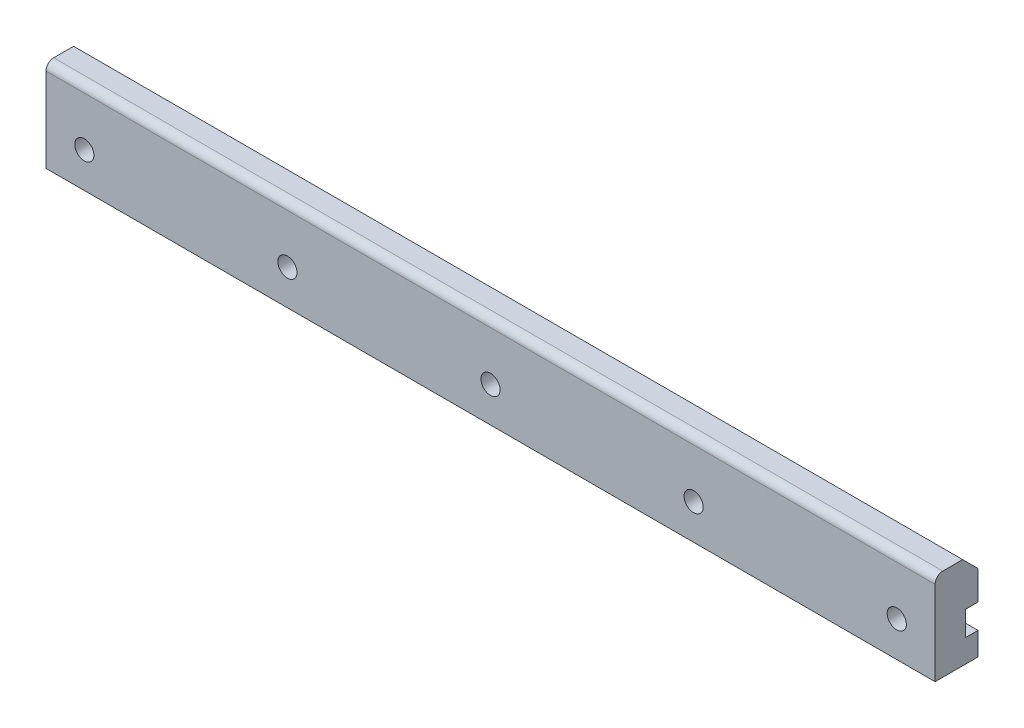
ISO-10303-21;
HEADER;
FILE_DESCRIPTION(('STEP AP214'),'2;1');
FILE_NAME('part.step','',(''),(''),'','','');
FILE_SCHEMA(('AUTOMOTIVE_DESIGN { 1 0 10303 214 1 1 1 1 }'));
ENDSEC;
DATA;
#1=APPLICATION_CONTEXT('core data for automotive mechanical design processes');
#2=APPLICATION_PROTOCOL_DEFINITION('international standard','automotive_design',2000,#1);
#3=PRODUCT_CONTEXT('',#1,'mechanical');
#4=PRODUCT('Part','Part','',(#3));
#5=PRODUCT_RELATED_PRODUCT_CATEGORY('part','',(#4));
#6=PRODUCT_DEFINITION_FORMATION('','',#4);
#7=PRODUCT_DEFINITION_CONTEXT('part definition',#1,'design');
#8=PRODUCT_DEFINITION('design','',#6,#7);
#9=PRODUCT_DEFINITION_SHAPE('','',#8);
#10=(LENGTH_UNIT() NAMED_UNIT(*) SI_UNIT(.MILLI.,.METRE.));
#11=(NAMED_UNIT(*) PLANE_ANGLE_UNIT() SI_UNIT($,.RADIAN.));
#12=(NAMED_UNIT(*) SI_UNIT($,.STERADIAN.) SOLID_ANGLE_UNIT());
#13=UNCERTAINTY_MEASURE_WITH_UNIT(LENGTH_MEASURE(1.E-05),#10,'distance_accuracy_value','');
#14=(GEOMETRIC_REPRESENTATION_CONTEXT(3) GLOBAL_UNCERTAINTY_ASSIGNED_CONTEXT((#13)) GLOBAL_UNIT_ASSIGNED_CONTEXT((#10,
#11,#12)) REPRESENTATION_CONTEXT('',''));
#15=CARTESIAN_POINT('',(0.,0.,0.));
#16=DIRECTION('',(0.,0.,1.));
#17=DIRECTION('',(1.,0.,0.));
#18=AXIS2_PLACEMENT_3D('',#15,#16,#17);
#19=CARTESIAN_POINT('',(0.,0.,0.));
#20=DIRECTION('',(0.,0.,1.));
#21=DIRECTION('',(1.,0.,0.));
#22=AXIS2_PLACEMENT_3D('',#19,#20,#21);
#23=PLANE('',#22);
#24=DIRECTION('',(0.,-1.,0.));
#25=VECTOR('',#24,1.);
#26=CARTESIAN_POINT('',(-290.,30.,0.));
#27=LINE('',#26,#25);
#28=CARTESIAN_POINT('',(-290.,-15.,0.));
#29=VERTEX_POINT('',#28);
#30=CARTESIAN_POINT('',(-290.,-30.,0.));
#31=VERTEX_POINT('',#30);
#32=EDGE_CURVE('E170',#29,#31,#27,.T.);
#33=ORIENTED_EDGE('',*,*,#32,.F.);
#34=DIRECTION('',(1.,0.,0.));
#35=VECTOR('',#34,1.);
#36=CARTESIAN_POINT('',(0.,-15.,0.));
#37=LINE('',#36,#35);
#38=CARTESIAN_POINT('',(290.,-15.,0.));
#39=VERTEX_POINT('',#38);
#40=EDGE_CURVE('E191',#29,#39,#37,.T.);
#41=ORIENTED_EDGE('',*,*,#40,.T.);
#42=DIRECTION('',(0.,1.,0.));
#43=VECTOR('',#42,1.);
#44=CARTESIAN_POINT('',(290.,30.,0.));
#45=LINE('',#44,#43);
#46=CARTESIAN_POINT('',(290.,-30.,0.));
#47=VERTEX_POINT('',#46);
#48=EDGE_CURVE('E165',#47,#39,#45,.T.);
#49=ORIENTED_EDGE('',*,*,#48,.F.);
#50=DIRECTION('',(1.,0.,0.));
#51=VECTOR('',#50,1.);
#52=CARTESIAN_POINT('',(-290.,-30.,0.));
#53=LINE('',#52,#51);
#54=EDGE_CURVE('E159',#31,#47,#53,.T.);
#55=ORIENTED_EDGE('',*,*,#54,.F.);
#56=EDGE_LOOP('',(#33,#41,#49,#55));
#57=FACE_BOUND('',#56,.T.);
#58=ADVANCED_FACE('F41',(#57),#23,.F.);
#59=CARTESIAN_POINT('',(290.,30.,28.));
#60=DIRECTION('',(-1.,0.,0.));
#61=DIRECTION('',(0.,0.,1.));
#62=AXIS2_PLACEMENT_3D('',#59,#60,#61);
#63=PLANE('',#62);
#64=CARTESIAN_POINT('',(290.,1.,0.));
#65=VERTEX_POINT('',#64);
#66=CARTESIAN_POINT('',(290.,20.,0.));
#67=VERTEX_POINT('',#66);
#68=EDGE_CURVE('E153',#65,#67,#45,.T.);
#69=ORIENTED_EDGE('',*,*,#68,.T.);
#70=DIRECTION('',(0.,-0.707106781186548,-0.707106781186548));
#71=VECTOR('',#70,1.);
#72=CARTESIAN_POINT('',(290.,30.,10.));
#73=LINE('',#72,#71);
#74=CARTESIAN_POINT('',(290.,30.,10.));
#75=VERTEX_POINT('',#74);
#76=EDGE_CURVE('E11',#67,#75,#73,.F.);
#77=ORIENTED_EDGE('',*,*,#76,.T.);
#78=DIRECTION('',(0.,0.,-1.));
#79=VECTOR('',#78,1.);
#80=CARTESIAN_POINT('',(290.,30.,28.));
#81=LINE('',#80,#79);
#82=CARTESIAN_POINT('',(290.,30.,23.));
#83=VERTEX_POINT('',#82);
#84=EDGE_CURVE('E180',#83,#75,#81,.T.);
#85=ORIENTED_EDGE('',*,*,#84,.F.);
#86=CARTESIAN_POINT('',(290.,25.,23.));
#87=DIRECTION('',(-1.,0.,0.));
#88=DIRECTION('',(0.,0.,1.));
#89=AXIS2_PLACEMENT_3D('',#86,#87,#88);
#90=CIRCLE('',#89,5.);
#91=CARTESIAN_POINT('',(290.,25.,28.));
#92=VERTEX_POINT('',#91);
#93=EDGE_CURVE('E190',#83,#92,#90,.F.);
#94=ORIENTED_EDGE('',*,*,#93,.T.);
#95=DIRECTION('',(0.,1.,0.));
#96=VECTOR('',#95,1.);
#97=CARTESIAN_POINT('',(290.,30.,28.));
#98=LINE('',#97,#96);
#99=CARTESIAN_POINT('',(290.,-30.,28.));
#100=VERTEX_POINT('',#99);
#101=EDGE_CURVE('E154',#100,#92,#98,.T.);
#102=ORIENTED_EDGE('',*,*,#101,.F.);
#103=DIRECTION('',(0.,0.,-1.));
#104=VECTOR('',#103,1.);
#105=CARTESIAN_POINT('',(290.,-30.,28.));
#106=LINE('',#105,#104);
#107=EDGE_CURVE('E161',#100,#47,#106,.T.);
#108=ORIENTED_EDGE('',*,*,#107,.T.);
#109=ORIENTED_EDGE('',*,*,#48,.T.);
#110=DIRECTION('',(0.,0.,-1.));
#111=VECTOR('',#110,1.);
#112=CARTESIAN_POINT('',(290.,-15.,8.));
#113=LINE('',#112,#111);
#114=CARTESIAN_POINT('',(290.,-15.,8.));
#115=VERTEX_POINT('',#114);
#116=EDGE_CURVE('E145',#115,#39,#113,.T.);
#117=ORIENTED_EDGE('',*,*,#116,.F.);
#118=DIRECTION('',(0.,-1.,0.));
#119=VECTOR('',#118,1.);
#120=CARTESIAN_POINT('',(290.,1.,8.));
#121=LINE('',#120,#119);
#122=CARTESIAN_POINT('',(290.,1.,8.));
#123=VERTEX_POINT('',#122);
#124=EDGE_CURVE('E144',#123,#115,#121,.T.);
#125=ORIENTED_EDGE('',*,*,#124,.F.);
#126=DIRECTION('',(0.,0.,1.));
#127=VECTOR('',#126,1.);
#128=CARTESIAN_POINT('',(290.,1.,8.));
#129=LINE('',#128,#127);
#130=EDGE_CURVE('E130',#65,#123,#129,.T.);
#131=ORIENTED_EDGE('',*,*,#130,.F.);
#132=EDGE_LOOP('',(#69,#77,#85,#94,#102,#108,#109,#117,#125,#131));
#133=FACE_BOUND('',#132,.T.);
#134=ADVANCED_FACE('F230',(#133),#63,.F.);
#135=CARTESIAN_POINT('',(-290.,30.,28.));
#136=DIRECTION('',(0.,-1.,0.));
#137=DIRECTION('',(0.,0.,-1.));
#138=AXIS2_PLACEMENT_3D('',#135,#136,#137);
#139=PLANE('',#138);
#140=ORIENTED_EDGE('',*,*,#84,.T.);
#141=DIRECTION('',(-1.,0.,0.));
#142=VECTOR('',#141,1.);
#143=CARTESIAN_POINT('',(-290.,30.,10.));
#144=LINE('',#143,#142);
#145=CARTESIAN_POINT('',(-290.,30.,10.));
#146=VERTEX_POINT('',#145);
#147=EDGE_CURVE('E193',#75,#146,#144,.T.);
#148=ORIENTED_EDGE('',*,*,#147,.T.);
#149=DIRECTION('',(0.,0.,-1.));
#150=VECTOR('',#149,1.);
#151=CARTESIAN_POINT('',(-290.,30.,28.));
#152=LINE('',#151,#150);
#153=CARTESIAN_POINT('',(-290.,30.,23.));
#154=VERTEX_POINT('',#153);
#155=EDGE_CURVE('E174',#154,#146,#152,.T.);
#156=ORIENTED_EDGE('',*,*,#155,.F.);
#157=DIRECTION('',(-1.,0.,0.));
#158=VECTOR('',#157,1.);
#159=CARTESIAN_POINT('',(290.,30.,23.));
#160=LINE('',#159,#158);
#161=EDGE_CURVE('E184',#154,#83,#160,.F.);
#162=ORIENTED_EDGE('',*,*,#161,.T.);
#163=EDGE_LOOP('',(#140,#148,#156,#162));
#164=FACE_BOUND('',#163,.T.);
#165=ADVANCED_FACE('F238',(#164),#139,.F.);
#166=CARTESIAN_POINT('',(-290.,30.,28.));
#167=DIRECTION('',(1.,0.,0.));
#168=DIRECTION('',(0.,0.,-1.));
#169=AXIS2_PLACEMENT_3D('',#166,#167,#168);
#170=PLANE('',#169);
#171=ORIENTED_EDGE('',*,*,#155,.T.);
#172=DIRECTION('',(0.,0.707106781186548,0.707106781186548));
#173=VECTOR('',#172,1.);
#174=CARTESIAN_POINT('',(-290.,30.,10.));
#175=LINE('',#174,#173);
#176=CARTESIAN_POINT('',(-290.,20.,0.));
#177=VERTEX_POINT('',#176);
#178=EDGE_CURVE('E66',#146,#177,#175,.F.);
#179=ORIENTED_EDGE('',*,*,#178,.T.);
#180=CARTESIAN_POINT('',(-290.,1.,0.));
#181=VERTEX_POINT('',#180);
#182=EDGE_CURVE('E142',#177,#181,#27,.T.);
#183=ORIENTED_EDGE('',*,*,#182,.T.);
#184=DIRECTION('',(0.,0.,1.));
#185=VECTOR('',#184,1.);
#186=CARTESIAN_POINT('',(-290.,1.,8.));
#187=LINE('',#186,#185);
#188=CARTESIAN_POINT('',(-290.,1.,8.));
#189=VERTEX_POINT('',#188);
#190=EDGE_CURVE('E121',#181,#189,#187,.T.);
#191=ORIENTED_EDGE('',*,*,#190,.T.);
#192=DIRECTION('',(0.,-1.,0.));
#193=VECTOR('',#192,1.);
#194=CARTESIAN_POINT('',(-290.,1.,8.));
#195=LINE('',#194,#193);
#196=CARTESIAN_POINT('',(-290.,-15.,8.));
#197=VERTEX_POINT('',#196);
#198=EDGE_CURVE('E134',#189,#197,#195,.T.);
#199=ORIENTED_EDGE('',*,*,#198,.T.);
#200=DIRECTION('',(0.,0.,-1.));
#201=VECTOR('',#200,1.);
#202=CARTESIAN_POINT('',(-290.,-15.,8.));
#203=LINE('',#202,#201);
#204=EDGE_CURVE('E135',#197,#29,#203,.T.);
#205=ORIENTED_EDGE('',*,*,#204,.T.);
#206=ORIENTED_EDGE('',*,*,#32,.T.);
#207=DIRECTION('',(0.,0.,-1.));
#208=VECTOR('',#207,1.);
#209=CARTESIAN_POINT('',(-290.,-30.,28.));
#210=LINE('',#209,#208);
#211=CARTESIAN_POINT('',(-290.,-30.,28.));
#212=VERTEX_POINT('',#211);
#213=EDGE_CURVE('E175',#212,#31,#210,.T.);
#214=ORIENTED_EDGE('',*,*,#213,.F.);
#215=DIRECTION('',(0.,-1.,0.));
#216=VECTOR('',#215,1.);
#217=CARTESIAN_POINT('',(-290.,30.,28.));
#218=LINE('',#217,#216);
#219=CARTESIAN_POINT('',(-290.,25.,28.));
#220=VERTEX_POINT('',#219);
#221=EDGE_CURVE('E156',#220,#212,#218,.T.);
#222=ORIENTED_EDGE('',*,*,#221,.F.);
#223=CARTESIAN_POINT('',(-290.,25.,23.));
#224=DIRECTION('',(1.,0.,0.));
#225=DIRECTION('',(0.,0.,-1.));
#226=AXIS2_PLACEMENT_3D('',#223,#224,#225);
#227=CIRCLE('',#226,5.);
#228=EDGE_CURVE('E182',#220,#154,#227,.F.);
#229=ORIENTED_EDGE('',*,*,#228,.T.);
#230=EDGE_LOOP('',(#171,#179,#183,#191,#199,#205,#206,#214,#222,#229));
#231=FACE_BOUND('',#230,.T.);
#232=ADVANCED_FACE('F137',(#231),#170,.F.);
#233=CARTESIAN_POINT('',(-290.,-30.,28.));
#234=DIRECTION('',(0.,1.,0.));
#235=DIRECTION('',(0.,0.,1.));
#236=AXIS2_PLACEMENT_3D('',#233,#234,#235);
#237=PLANE('',#236);
#238=ORIENTED_EDGE('',*,*,#54,.T.);
#239=ORIENTED_EDGE('',*,*,#107,.F.);
#240=DIRECTION('',(1.,0.,0.));
#241=VECTOR('',#240,1.);
#242=CARTESIAN_POINT('',(-290.,-30.,28.));
#243=LINE('',#242,#241);
#244=EDGE_CURVE('E163',#212,#100,#243,.T.);
#245=ORIENTED_EDGE('',*,*,#244,.F.);
#246=ORIENTED_EDGE('',*,*,#213,.T.);
#247=EDGE_LOOP('',(#238,#239,#245,#246));
#248=FACE_BOUND('',#247,.T.);
#249=ADVANCED_FACE('F251',(#248),#237,.F.);
#250=CARTESIAN_POINT('',(0.,0.,28.));
#251=DIRECTION('',(0.,0.,1.));
#252=DIRECTION('',(1.,0.,0.));
#253=AXIS2_PLACEMENT_3D('',#250,#251,#252);
#254=PLANE('',#253);
#255=CARTESIAN_POINT('',(-265.,-7.,28.));
#256=DIRECTION('',(0.,0.,1.));
#257=DIRECTION('',(1.,0.,0.));
#258=AXIS2_PLACEMENT_3D('',#255,#256,#257);
#259=CIRCLE('',#258,6.25);
#260=CARTESIAN_POINT('',(-258.75,-7.,28.));
#261=VERTEX_POINT('',#260);
#262=EDGE_CURVE('E201',#261,#261,#259,.T.);
#263=ORIENTED_EDGE('',*,*,#262,.F.);
#264=EDGE_LOOP('',(#263));
#265=FACE_BOUND('',#264,.T.);
#266=CARTESIAN_POINT('',(-132.5,-7.,28.));
#267=DIRECTION('',(0.,0.,1.));
#268=DIRECTION('',(1.,0.,0.));
#269=AXIS2_PLACEMENT_3D('',#266,#267,#268);
#270=CIRCLE('',#269,6.25);
#271=CARTESIAN_POINT('',(-126.25,-7.,28.));
#272=VERTEX_POINT('',#271);
#273=EDGE_CURVE('E308',#272,#272,#270,.T.);
#274=ORIENTED_EDGE('',*,*,#273,.F.);
#275=EDGE_LOOP('',(#274));
#276=FACE_BOUND('',#275,.T.);
#277=CARTESIAN_POINT('',(0.,-7.,28.));
#278=DIRECTION('',(0.,0.,1.));
#279=DIRECTION('',(1.,0.,0.));
#280=AXIS2_PLACEMENT_3D('',#277,#278,#279);
#281=CIRCLE('',#280,6.25);
#282=CARTESIAN_POINT('',(6.25000000000006,-7.,28.));
#283=VERTEX_POINT('',#282);
#284=EDGE_CURVE('E304',#283,#283,#281,.T.);
#285=ORIENTED_EDGE('',*,*,#284,.F.);
#286=EDGE_LOOP('',(#285));
#287=FACE_BOUND('',#286,.T.);
#288=CARTESIAN_POINT('',(132.5,-7.,28.));
#289=DIRECTION('',(0.,0.,1.));
#290=DIRECTION('',(1.,0.,0.));
#291=AXIS2_PLACEMENT_3D('',#288,#289,#290);
#292=CIRCLE('',#291,6.25);
#293=CARTESIAN_POINT('',(138.75,-7.,28.));
#294=VERTEX_POINT('',#293);
#295=EDGE_CURVE('E303',#294,#294,#292,.T.);
#296=ORIENTED_EDGE('',*,*,#295,.F.);
#297=EDGE_LOOP('',(#296));
#298=FACE_BOUND('',#297,.T.);
#299=CARTESIAN_POINT('',(265.,-7.,28.));
#300=DIRECTION('',(0.,0.,1.));
#301=DIRECTION('',(1.,0.,0.));
#302=AXIS2_PLACEMENT_3D('',#299,#300,#301);
#303=CIRCLE('',#302,6.25);
#304=CARTESIAN_POINT('',(271.25,-7.,28.));
#305=VERTEX_POINT('',#304);
#306=EDGE_CURVE('E150',#305,#305,#303,.T.);
#307=ORIENTED_EDGE('',*,*,#306,.F.);
#308=EDGE_LOOP('',(#307));
#309=FACE_BOUND('',#308,.T.);
#310=ORIENTED_EDGE('',*,*,#101,.T.);
#311=DIRECTION('',(-1.,0.,0.));
#312=VECTOR('',#311,1.);
#313=CARTESIAN_POINT('',(-290.,25.,28.));
#314=LINE('',#313,#312);
#315=EDGE_CURVE('E179',#92,#220,#314,.T.);
#316=ORIENTED_EDGE('',*,*,#315,.T.);
#317=ORIENTED_EDGE('',*,*,#221,.T.);
#318=ORIENTED_EDGE('',*,*,#244,.T.);
#319=EDGE_LOOP('',(#310,#316,#317,#318));
#320=FACE_BOUND('',#319,.T.);
#321=ADVANCED_FACE('F246',(#265,#276,#287,#298,#309,#320),#254,.T.);
#322=ORIENTED_EDGE('',*,*,#182,.F.);
#323=DIRECTION('',(1.,0.,0.));
#324=VECTOR('',#323,1.);
#325=CARTESIAN_POINT('',(0.,20.,0.));
#326=LINE('',#325,#324);
#327=EDGE_CURVE('E51',#177,#67,#326,.T.);
#328=ORIENTED_EDGE('',*,*,#327,.T.);
#329=ORIENTED_EDGE('',*,*,#68,.F.);
#330=DIRECTION('',(-1.,0.,0.));
#331=VECTOR('',#330,1.);
#332=CARTESIAN_POINT('',(0.,1.,0.));
#333=LINE('',#332,#331);
#334=EDGE_CURVE('E186',#65,#181,#333,.T.);
#335=ORIENTED_EDGE('',*,*,#334,.T.);
#336=EDGE_LOOP('',(#322,#328,#329,#335));
#337=FACE_BOUND('',#336,.T.);
#338=ADVANCED_FACE('F235',(#337),#23,.F.);
#339=CARTESIAN_POINT('',(0.,25.,23.));
#340=DIRECTION('',(1.,0.,0.));
#341=DIRECTION('',(0.,0.,-1.));
#342=AXIS2_PLACEMENT_3D('',#339,#340,#341);
#343=CYLINDRICAL_SURFACE('',#342,5.);
#344=ORIENTED_EDGE('',*,*,#93,.F.);
#345=ORIENTED_EDGE('',*,*,#161,.F.);
#346=ORIENTED_EDGE('',*,*,#228,.F.);
#347=ORIENTED_EDGE('',*,*,#315,.F.);
#348=EDGE_LOOP('',(#344,#345,#346,#347));
#349=FACE_BOUND('',#348,.T.);
#350=ADVANCED_FACE('F244',(#349),#343,.T.);
#351=CARTESIAN_POINT('',(-290.,-15.,8.));
#352=DIRECTION('',(0.,-1.,0.));
#353=DIRECTION('',(0.,0.,-1.));
#354=AXIS2_PLACEMENT_3D('',#351,#352,#353);
#355=PLANE('',#354);
#356=ORIENTED_EDGE('',*,*,#204,.F.);
#357=DIRECTION('',(1.,0.,0.));
#358=VECTOR('',#357,1.);
#359=CARTESIAN_POINT('',(-290.,-15.,8.));
#360=LINE('',#359,#358);
#361=EDGE_CURVE('E131',#197,#115,#360,.T.);
#362=ORIENTED_EDGE('',*,*,#361,.T.);
#363=ORIENTED_EDGE('',*,*,#116,.T.);
#364=ORIENTED_EDGE('',*,*,#40,.F.);
#365=EDGE_LOOP('',(#356,#362,#363,#364));
#366=FACE_BOUND('',#365,.T.);
#367=ADVANCED_FACE('F252',(#366),#355,.F.);
#368=CARTESIAN_POINT('',(-290.,1.,8.));
#369=DIRECTION('',(0.,1.,0.));
#370=DIRECTION('',(0.,0.,1.));
#371=AXIS2_PLACEMENT_3D('',#368,#369,#370);
#372=PLANE('',#371);
#373=ORIENTED_EDGE('',*,*,#130,.T.);
#374=DIRECTION('',(1.,0.,0.));
#375=VECTOR('',#374,1.);
#376=CARTESIAN_POINT('',(-290.,1.,8.));
#377=LINE('',#376,#375);
#378=EDGE_CURVE('E119',#189,#123,#377,.T.);
#379=ORIENTED_EDGE('',*,*,#378,.F.);
#380=ORIENTED_EDGE('',*,*,#190,.F.);
#381=ORIENTED_EDGE('',*,*,#334,.F.);
#382=EDGE_LOOP('',(#373,#379,#380,#381));
#383=FACE_BOUND('',#382,.T.);
#384=ADVANCED_FACE('F125',(#383),#372,.F.);
#385=CARTESIAN_POINT('',(-290.,1.,8.));
#386=DIRECTION('',(0.,0.,1.));
#387=DIRECTION('',(0.,-1.,0.));
#388=AXIS2_PLACEMENT_3D('',#385,#386,#387);
#389=PLANE('',#388);
#390=CARTESIAN_POINT('',(-265.,-7.,8.));
#391=DIRECTION('',(0.,0.,1.));
#392=DIRECTION('',(0.,-1.,0.));
#393=AXIS2_PLACEMENT_3D('',#390,#391,#392);
#394=CIRCLE('',#393,6.25);
#395=CARTESIAN_POINT('',(-265.,-13.25,8.));
#396=VERTEX_POINT('',#395);
#397=EDGE_CURVE('E46',#396,#396,#394,.T.);
#398=ORIENTED_EDGE('',*,*,#397,.T.);
#399=EDGE_LOOP('',(#398));
#400=FACE_BOUND('',#399,.T.);
#401=CARTESIAN_POINT('',(-132.5,-7.,8.));
#402=DIRECTION('',(0.,0.,1.));
#403=DIRECTION('',(0.,-1.,0.));
#404=AXIS2_PLACEMENT_3D('',#401,#402,#403);
#405=CIRCLE('',#404,6.25);
#406=CARTESIAN_POINT('',(-132.5,-13.25,8.));
#407=VERTEX_POINT('',#406);
#408=EDGE_CURVE('E206',#407,#407,#405,.T.);
#409=ORIENTED_EDGE('',*,*,#408,.T.);
#410=EDGE_LOOP('',(#409));
#411=FACE_BOUND('',#410,.T.);
#412=CARTESIAN_POINT('',(0.,-7.,8.));
#413=DIRECTION('',(0.,0.,1.));
#414=DIRECTION('',(0.,-1.,0.));
#415=AXIS2_PLACEMENT_3D('',#412,#413,#414);
#416=CIRCLE('',#415,6.25);
#417=CARTESIAN_POINT('',(0.,-13.25,8.));
#418=VERTEX_POINT('',#417);
#419=EDGE_CURVE('E207',#418,#418,#416,.T.);
#420=ORIENTED_EDGE('',*,*,#419,.T.);
#421=EDGE_LOOP('',(#420));
#422=FACE_BOUND('',#421,.T.);
#423=CARTESIAN_POINT('',(132.5,-7.,8.));
#424=DIRECTION('',(0.,0.,1.));
#425=DIRECTION('',(0.,-1.,0.));
#426=AXIS2_PLACEMENT_3D('',#423,#424,#425);
#427=CIRCLE('',#426,6.25);
#428=CARTESIAN_POINT('',(132.5,-13.25,8.));
#429=VERTEX_POINT('',#428);
#430=EDGE_CURVE('E205',#429,#429,#427,.T.);
#431=ORIENTED_EDGE('',*,*,#430,.T.);
#432=EDGE_LOOP('',(#431));
#433=FACE_BOUND('',#432,.T.);
#434=CARTESIAN_POINT('',(265.,-7.,8.));
#435=DIRECTION('',(0.,0.,1.));
#436=DIRECTION('',(0.,-1.,0.));
#437=AXIS2_PLACEMENT_3D('',#434,#435,#436);
#438=CIRCLE('',#437,6.25);
#439=CARTESIAN_POINT('',(265.,-13.25,8.));
#440=VERTEX_POINT('',#439);
#441=EDGE_CURVE('E197',#440,#440,#438,.T.);
#442=ORIENTED_EDGE('',*,*,#441,.T.);
#443=EDGE_LOOP('',(#442));
#444=FACE_BOUND('',#443,.T.);
#445=ORIENTED_EDGE('',*,*,#124,.T.);
#446=ORIENTED_EDGE('',*,*,#361,.F.);
#447=ORIENTED_EDGE('',*,*,#198,.F.);
#448=ORIENTED_EDGE('',*,*,#378,.T.);
#449=EDGE_LOOP('',(#445,#446,#447,#448));
#450=FACE_BOUND('',#449,.T.);
#451=ADVANCED_FACE('F138',(#400,#411,#422,#433,#444,#450),#389,.F.);
#452=CARTESIAN_POINT('',(-290.,30.,10.));
#453=DIRECTION('',(0.,-0.707106781186547,0.707106781186547));
#454=DIRECTION('',(-1.,0.,0.));
#455=AXIS2_PLACEMENT_3D('',#452,#453,#454);
#456=PLANE('',#455);
#457=ORIENTED_EDGE('',*,*,#76,.F.);
#458=ORIENTED_EDGE('',*,*,#327,.F.);
#459=ORIENTED_EDGE('',*,*,#178,.F.);
#460=ORIENTED_EDGE('',*,*,#147,.F.);
#461=EDGE_LOOP('',(#457,#458,#459,#460));
#462=FACE_BOUND('',#461,.T.);
#463=ADVANCED_FACE('F42',(#462),#456,.F.);
#464=CARTESIAN_POINT('',(265.,-7.,0.));
#465=DIRECTION('',(0.,0.,1.));
#466=DIRECTION('',(1.,0.,0.));
#467=AXIS2_PLACEMENT_3D('',#464,#465,#466);
#468=CYLINDRICAL_SURFACE('',#467,6.25);
#469=ORIENTED_EDGE('',*,*,#306,.T.);
#470=EDGE_LOOP('',(#469));
#471=FACE_BOUND('',#470,.T.);
#472=ORIENTED_EDGE('',*,*,#441,.F.);
#473=EDGE_LOOP('',(#472));
#474=FACE_BOUND('',#473,.T.);
#475=ADVANCED_FACE('F283',(#471,#474),#468,.F.);
#476=CARTESIAN_POINT('',(132.5,-7.,0.));
#477=DIRECTION('',(0.,0.,1.));
#478=DIRECTION('',(1.,0.,0.));
#479=AXIS2_PLACEMENT_3D('',#476,#477,#478);
#480=CYLINDRICAL_SURFACE('',#479,6.25);
#481=ORIENTED_EDGE('',*,*,#295,.T.);
#482=EDGE_LOOP('',(#481));
#483=FACE_BOUND('',#482,.T.);
#484=ORIENTED_EDGE('',*,*,#430,.F.);
#485=EDGE_LOOP('',(#484));
#486=FACE_BOUND('',#485,.T.);
#487=ADVANCED_FACE('F293',(#483,#486),#480,.F.);
#488=CARTESIAN_POINT('',(0.,-7.,0.));
#489=DIRECTION('',(0.,0.,1.));
#490=DIRECTION('',(1.,0.,0.));
#491=AXIS2_PLACEMENT_3D('',#488,#489,#490);
#492=CYLINDRICAL_SURFACE('',#491,6.25);
#493=ORIENTED_EDGE('',*,*,#284,.T.);
#494=EDGE_LOOP('',(#493));
#495=FACE_BOUND('',#494,.T.);
#496=ORIENTED_EDGE('',*,*,#419,.F.);
#497=EDGE_LOOP('',(#496));
#498=FACE_BOUND('',#497,.T.);
#499=ADVANCED_FACE('F224',(#495,#498),#492,.F.);
#500=CARTESIAN_POINT('',(-132.5,-7.,0.));
#501=DIRECTION('',(0.,0.,1.));
#502=DIRECTION('',(1.,0.,0.));
#503=AXIS2_PLACEMENT_3D('',#500,#501,#502);
#504=CYLINDRICAL_SURFACE('',#503,6.25);
#505=ORIENTED_EDGE('',*,*,#273,.T.);
#506=EDGE_LOOP('',(#505));
#507=FACE_BOUND('',#506,.T.);
#508=ORIENTED_EDGE('',*,*,#408,.F.);
#509=EDGE_LOOP('',(#508));
#510=FACE_BOUND('',#509,.T.);
#511=ADVANCED_FACE('F218',(#507,#510),#504,.F.);
#512=CARTESIAN_POINT('',(-265.,-7.,0.));
#513=DIRECTION('',(0.,0.,1.));
#514=DIRECTION('',(1.,0.,0.));
#515=AXIS2_PLACEMENT_3D('',#512,#513,#514);
#516=CYLINDRICAL_SURFACE('',#515,6.25);
#517=ORIENTED_EDGE('',*,*,#262,.T.);
#518=EDGE_LOOP('',(#517));
#519=FACE_BOUND('',#518,.T.);
#520=ORIENTED_EDGE('',*,*,#397,.F.);
#521=EDGE_LOOP('',(#520));
#522=FACE_BOUND('',#521,.T.);
#523=ADVANCED_FACE('F216',(#519,#522),#516,.F.);
#524=CLOSED_SHELL('',(#58,#134,#165,#232,#249,#321,#338,#350,#367,#384,#451,#463,#475,#487,#499,
#511,#523));
#525=MANIFOLD_SOLID_BREP('B2',#524);
#526=ADVANCED_BREP_SHAPE_REPRESENTATION('',(#18,#525),#14);
#527=SHAPE_DEFINITION_REPRESENTATION(#9,#526);
ENDSEC;
END-ISO-10303-21;
